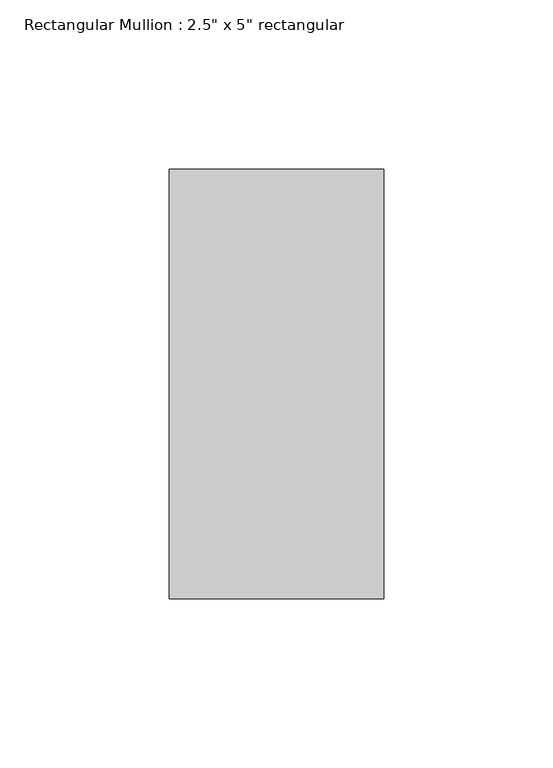
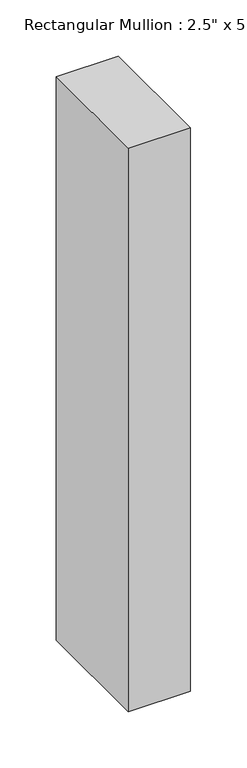
"""IFC4 building model written with IfcOpenShell, lengths in millimetres: member geometry."""

from ifc_helpers import new_model, si_unit, frame, origin, place, context, project, spatial, polyline, outline, extrude, source, transform, mapped, element, save


def member_47bfaf8a(model_context):
    return source(origin(), model_context, "Body", "SweptSolid", [
        extrude(outline(polyline([(0.0, 63.5), (0.0, -63.5), (-63.5, -63.5), (-63.5, 63.5), (0.0, 63.5)])), frame((0.0, 0.0, -609.6), z_axis=(0.0, 0.0, 1.0), x_axis=(1.0, 0.0, 0.0)), (0.0, 0.0, 1.0), 609.6),
    ])


if __name__ == "__main__":
    model = new_model("IFC4")
    model_context = context("Model", 3, world=origin())
    ifc_project = project(units=[si_unit("LENGTHUNIT", "METRE", prefix="MILLI")], contexts=[model_context])
    site = spatial("IfcSite", under=ifc_project)
    building = spatial("IfcBuilding", under=site)
    placement = place(None, origin())
    member_shape = member_47bfaf8a(model_context)
    element("IfcMember", 1, ObjectType="Rectangular Mullion : 2.5\" x 5\" rectangular", at=placement, inside=building, context=model_context, shape_type="MappedRepresentation", body=[
        mapped(member_shape, transform((0.0, 0.0, 0.0), x_axis=(1.0, 0.0, 0.0), y_axis=(0.0, 1.0, 0.0), z_axis=(0.0, 0.0, 1.0))),
    ])
    save(model, "model.ifc")

# Revit data of these elements
# Type "Rectangular Mullion : 2.5\" x 5\" rectangular"
#   built-in parameter 1007304 = 0.416667 (stored number, unit not read)
#   built-in parameter 1007301 = 0.104167 (stored number, unit not read)
#   built-in parameter 1007300 = 0.104167 (stored number, unit not read)
# Element 1 (IfcMember, "Rectangular Mullion : 2.5\" x 5\" rectangular")
#   Materials on its faces: "Iron, Ductile"
# Materials
#   "Iron, Ductile": class "Metal", colour RGB 0 0 0, transparency 0, Description = "Ductile cast iron", Cost = 0
